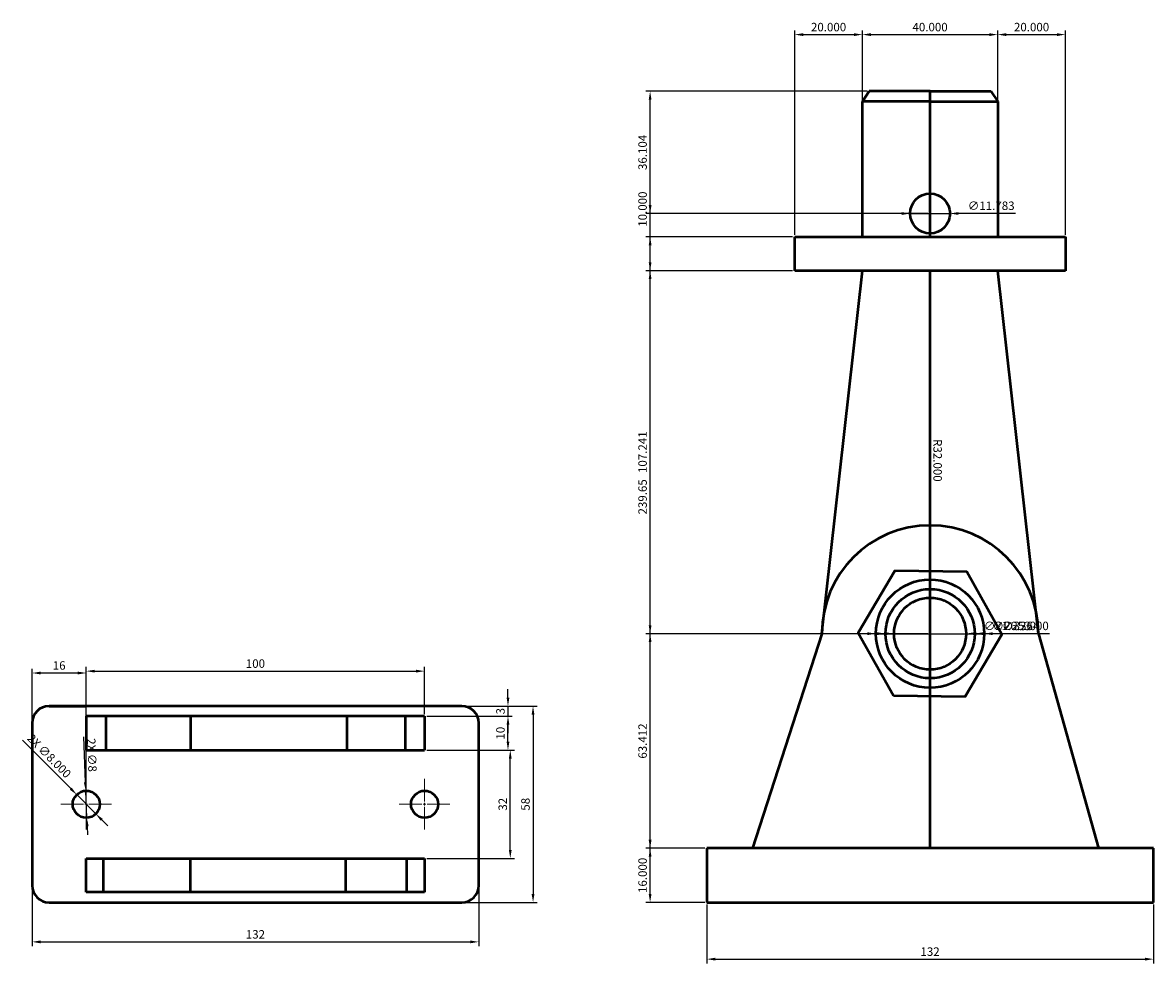
# Model space of a CAD drawing. Units: millimetres. Extents: x 1132 to 1696, y 1793 to 2376.
# Tile 3 of 4: x 1150 to 1484, y 2098 to 2376. Entities that reach past the tile are written whole.
import ezdxf

# ---------------------------------------------------------------- set-up
doc = ezdxf.new("R2010")
doc.units = ezdxf.units.MM
doc.linetypes.add('CENTER2', pattern=[28.575, 19.05, -3.175, 3.175, -3.175])
for name, color, linetype, lineweight in [('M-CNTR', 1, 'CENTER2', 18), ('M-DIMS', 2, 'Continuous', 25), ('M-OUTL', 7, 'Continuous', 50)]:
    doc.layers.add(name, color=color, linetype=linetype, lineweight=lineweight)
doc.styles.get("Standard").update_dxf_attribs({"font": 'arial.ttf'})
doc.dimstyles.new('ISO-25', dxfattribs={"dimtxt": 2.5, "dimasz": 2.5, "dimexe": 1.25, "dimexo": 0.625, "dimtad": 1, "dimtxsty": 'Standard', "dimcen": 2.5, "dimadec": 0, "dimazin": 0, "dimtfac": 1, "dimtmove": 0, "dimatfit": 3, "dimfxl": 1, "dimarcsym": 0})

# ---------------------------------------------------------------- blocks, each defined once
blk = doc.blocks.new('*D1')
at = {"layer": 'Defpoints', "color": 0, "transparency": 16777216}
for p in [(1152.81, 2120.87), (1284.81, 2120.87), (1284.81, 2104.21)]:
    blk.add_point(p, dxfattribs=at)
at = {"layer": 'M-DIMS', "color": 0, "lineweight": -2, "transparency": 16777216}
for p, q in [((1152.81, 2120.25), (1152.81, 2102.96)), ((1284.81, 2120.25), (1284.81, 2102.96)), ((1155.31, 2104.21), (1282.31, 2104.21))]:
    blk.add_line(p, q, dxfattribs=at)
at = {"layer": 'M-DIMS', "color": 0, "transparency": 16777216}
for points in [[(1155.31, 2104.63), (1155.31, 2103.79), (1152.81, 2104.21)], [(1282.31, 2104.63), (1282.31, 2103.79), (1284.81, 2104.21)]]:
    blk.add_solid(points, dxfattribs=at)
at = {"layer": 'M-DIMS', "color": 0, "transparency": 16777216, "insert": (1218.81, 2106.11), "char_height": 2.5, "attachment_point": 5}
blk.add_mtext('132', dxfattribs=at)
blk = doc.blocks.new('*D2')
at = {"layer": 'Defpoints', "color": 0, "transparency": 16777216}
for p in [(1279.81, 2173.87), (1279.81, 2115.87), (1300.87, 2115.87)]:
    blk.add_point(p, dxfattribs=at)
at = {"layer": 'M-DIMS', "color": 0, "lineweight": -2, "transparency": 16777216}
for p, q in [((1280.43, 2173.87), (1302.12, 2173.87)), ((1300.87, 2171.37), (1300.87, 2118.37)), ((1280.43, 2115.87), (1302.12, 2115.87))]:
    blk.add_line(p, q, dxfattribs=at)
at = {"layer": 'M-DIMS', "color": 0, "transparency": 16777216}
for points in [[(1300.45, 2171.37), (1301.28, 2171.37), (1300.87, 2173.87)], [(1300.45, 2118.37), (1301.28, 2118.37), (1300.87, 2115.87)]]:
    blk.add_solid(points, dxfattribs=at)
at = {"layer": 'M-DIMS', "color": 0, "transparency": 16777216, "insert": (1298.96, 2144.87), "char_height": 2.5, "attachment_point": 5, "rotation": 90}
blk.add_mtext('58', dxfattribs=at)
blk = doc.blocks.new('*D3')
at = {"layer": 'Defpoints', "color": 0, "transparency": 16777216}
for p in [(1268.81, 2160.87), (1294.14, 2160.87), (1268.81, 2128.87)]:
    blk.add_point(p, dxfattribs=at)
at = {"layer": 'M-DIMS', "color": 0, "lineweight": -2, "transparency": 16777216}
for p, q in [((1269.43, 2160.87), (1295.39, 2160.87)), ((1294.14, 2131.37), (1294.14, 2158.37)), ((1269.43, 2128.87), (1295.39, 2128.87))]:
    blk.add_line(p, q, dxfattribs=at)
at = {"layer": 'M-DIMS', "color": 0, "transparency": 16777216}
for points in [[(1293.72, 2158.37), (1294.55, 2158.37), (1294.14, 2160.87)], [(1293.72, 2131.37), (1294.55, 2131.37), (1294.14, 2128.87)]]:
    blk.add_solid(points, dxfattribs=at)
at = {"layer": 'M-DIMS', "color": 0, "transparency": 16777216, "insert": (1292.24, 2144.87), "char_height": 2.5, "attachment_point": 5, "rotation": 90}
blk.add_mtext('32', dxfattribs=at)
blk = doc.blocks.new('*D4')
at = {"layer": 'Defpoints', "color": 0, "transparency": 16777216}
for p in [(1268.81, 2170.87), (1293.46, 2170.87), (1268.81, 2160.87)]:
    blk.add_point(p, dxfattribs=at)
at = {"layer": 'M-DIMS', "color": 0, "lineweight": -2, "transparency": 16777216}
for p, q in [((1269.43, 2170.87), (1294.71, 2170.87)), ((1293.46, 2163.37), (1293.46, 2168.37)), ((1269.43, 2160.87), (1294.71, 2160.87))]:
    blk.add_line(p, q, dxfattribs=at)
at = {"layer": 'M-DIMS', "color": 0, "transparency": 16777216}
for points in [[(1293.05, 2168.37), (1293.88, 2168.37), (1293.46, 2170.87)], [(1293.05, 2163.37), (1293.88, 2163.37), (1293.46, 2160.87)]]:
    blk.add_solid(points, dxfattribs=at)
at = {"layer": 'M-DIMS', "color": 0, "transparency": 16777216, "insert": (1291.56, 2165.87), "char_height": 2.5, "attachment_point": 5, "rotation": 90}
blk.add_mtext('10', dxfattribs=at)
blk = doc.blocks.new('*D5')
at = {"layer": 'Defpoints', "color": 0, "transparency": 16777216}
for p in [(1279.81, 2173.87), (1282.07, 2170.87), (1293.46, 2170.87)]:
    blk.add_point(p, dxfattribs=at)
at = {"layer": 'M-DIMS', "color": 0, "lineweight": -2, "transparency": 16777216}
for p, q in [((1293.46, 2176.37), (1293.46, 2178.87)), ((1280.43, 2173.87), (1294.71, 2173.87)), ((1293.46, 2173.87), (1293.46, 2170.87)), ((1282.7, 2170.87), (1294.71, 2170.87)), ((1293.46, 2168.37), (1293.46, 2165.87))]:
    blk.add_line(p, q, dxfattribs=at)
at = {"layer": 'M-DIMS', "color": 0, "transparency": 16777216}
for points in [[(1293.05, 2176.37), (1293.88, 2176.37), (1293.46, 2173.87)], [(1293.05, 2168.37), (1293.88, 2168.37), (1293.46, 2170.87)]]:
    blk.add_solid(points, dxfattribs=at)
at = {"layer": 'M-DIMS', "color": 0, "transparency": 16777216, "insert": (1291.56, 2172.37), "char_height": 2.5, "attachment_point": 5, "rotation": 90}
blk.add_mtext('3', dxfattribs=at)
blk = doc.blocks.new('*D6')
at = {"layer": 'Defpoints', "color": 0, "transparency": 16777216}
for p in [(1268.81, 2184.2), (1168.81, 2170.87), (1268.81, 2170.87)]:
    blk.add_point(p, dxfattribs=at)
at = {"layer": 'M-DIMS', "color": 0, "lineweight": -2, "transparency": 16777216}
for p, q in [((1168.81, 2171.5), (1168.81, 2185.45)), ((1171.31, 2184.2), (1266.31, 2184.2)), ((1268.81, 2171.5), (1268.81, 2185.45))]:
    blk.add_line(p, q, dxfattribs=at)
at = {"layer": 'M-DIMS', "color": 0, "transparency": 16777216}
for points in [[(1171.31, 2184.61), (1171.31, 2183.78), (1168.81, 2184.2)], [(1266.31, 2184.61), (1266.31, 2183.78), (1268.81, 2184.2)]]:
    blk.add_solid(points, dxfattribs=at)
at = {"layer": 'M-DIMS', "color": 0, "transparency": 16777216, "insert": (1218.81, 2186.1), "char_height": 2.5, "attachment_point": 5}
blk.add_mtext('100', dxfattribs=at)
blk = doc.blocks.new('*D7')
at = {"layer": 'Defpoints', "color": 0, "transparency": 16777216}
for p in [(1152.81, 2183.65), (1152.81, 2144.87), (1168.81, 2144.87)]:
    blk.add_point(p, dxfattribs=at)
at = {"layer": 'M-DIMS', "color": 0, "lineweight": -2, "transparency": 16777216}
for p, q in [((1152.81, 2145.5), (1152.81, 2184.9)), ((1166.31, 2183.65), (1155.31, 2183.65)), ((1168.81, 2145.5), (1168.81, 2184.9))]:
    blk.add_line(p, q, dxfattribs=at)
at = {"layer": 'M-DIMS', "color": 0, "transparency": 16777216}
for points in [[(1155.31, 2184.06), (1155.31, 2183.23), (1152.81, 2183.65)], [(1166.31, 2184.06), (1166.31, 2183.23), (1168.81, 2183.65)]]:
    blk.add_solid(points, dxfattribs=at)
at = {"layer": 'M-DIMS', "color": 0, "transparency": 16777216, "insert": (1160.81, 2185.55), "char_height": 2.5, "attachment_point": 5}
blk.add_mtext('16', dxfattribs=at)
blk = doc.blocks.new('*U8')
at = {"layer": 'M-CNTR', "color": 0, "transparency": 16777216}
for p, q in [((0, 0.8), (0, 7.5)), ((-7.5, 0), (-0.8, 0)), ((0.8, 0), (7.5, 0)), ((0, -7.5), (0, -0.8))]:
    blk.add_line(p, q, dxfattribs=at)
at = {"layer": 'M-CNTR', "color": 0, "linetype": 'Continuous', "transparency": 16777216}
for p, q in [((-0.4, 0), (0.4, 0)), ((0, -0.4), (0, 0.4))]:
    blk.add_line(p, q, dxfattribs=at)
blk = doc.blocks.new('*U9')
at = {"layer": 'M-CNTR', "color": 0, "transparency": 16777216}
for p, q in [((0, 0.8), (0, 7.5)), ((-7.5, 0), (-0.8, 0)), ((0.8, 0), (7.5, 0)), ((0, -7.5), (0, -0.8))]:
    blk.add_line(p, q, dxfattribs=at)
at = {"layer": 'M-CNTR', "color": 0, "linetype": 'Continuous', "transparency": 16777216}
for p, q in [((-0.4, 0), (0.4, 0)), ((0, -0.4), (0, 0.4))]:
    blk.add_line(p, q, dxfattribs=at)
blk = doc.blocks.new('*D35')
at = {"layer": 'Defpoints', "color": 0, "transparency": 16777216}
for p in [(1352.22, 2115.86), (1484.22, 2115.86), (1484.22, 2099.11)]:
    blk.add_point(p, dxfattribs=at)
at = {"layer": 'M-DIMS', "color": 0, "lineweight": -2, "transparency": 16777216}
for p, q in [((1352.22, 2115.23), (1352.22, 2097.86)), ((1484.22, 2115.23), (1484.22, 2097.86)), ((1354.72, 2099.11), (1481.72, 2099.11))]:
    blk.add_line(p, q, dxfattribs=at)
at = {"layer": 'M-DIMS', "color": 0, "transparency": 16777216}
for points in [[(1354.72, 2099.53), (1354.72, 2098.69), (1352.22, 2099.11)], [(1481.72, 2099.53), (1481.72, 2098.69), (1484.22, 2099.11)]]:
    blk.add_solid(points, dxfattribs=at)
at = {"layer": 'M-DIMS', "color": 0, "transparency": 16777216, "insert": (1418.22, 2101.01), "char_height": 2.5, "attachment_point": 5}
blk.add_mtext('132', dxfattribs=at)
blk = doc.blocks.new('*D36')
at = {"layer": 'Defpoints', "color": 0, "transparency": 16777216}
for p in [(1335.47, 2355.51), (1400.22, 2355.51), (1352.22, 2115.86)]:
    blk.add_point(p, dxfattribs=at)
at = {"layer": 'M-DIMS', "color": 0, "lineweight": -2, "transparency": 16777216}
for p, q in [((1399.6, 2355.51), (1334.22, 2355.51)), ((1335.47, 2118.36), (1335.47, 2353.01)), ((1351.6, 2115.86), (1334.22, 2115.86))]:
    blk.add_line(p, q, dxfattribs=at)
at = {"layer": 'M-DIMS', "color": 0, "transparency": 16777216}
for points in [[(1335.06, 2353.01), (1335.89, 2353.01), (1335.47, 2355.51)], [(1335.06, 2118.36), (1335.89, 2118.36), (1335.47, 2115.86)]]:
    blk.add_solid(points, dxfattribs=at)
at = {"layer": 'M-DIMS', "color": 0, "transparency": 16777216, "insert": (1333.57, 2235.69), "char_height": 2.5, "attachment_point": 5, "rotation": 90}
blk.add_mtext('239.65', dxfattribs=at)
blk = doc.blocks.new('*D49')
at = {"layer": 'Defpoints', "color": 0, "transparency": 16777216}
for p in [(1168.64, 2148.87), (1168.98, 2140.88)]:
    blk.add_point(p, dxfattribs=at)
at = {"layer": 'M-DIMS', "color": 0, "lineweight": -2, "transparency": 16777216}
for p, q in [((1167.95, 2164.75), (1168.53, 2151.37)), ((1168.98, 2140.88), (1168.64, 2148.87)), ((1169.09, 2138.38), (1169.2, 2135.88))]:
    blk.add_line(p, q, dxfattribs=at)
at = {"layer": 'M-DIMS', "color": 0, "transparency": 16777216}
for points in [[(1168.94, 2151.39), (1168.11, 2151.35), (1168.64, 2148.87)], [(1169.51, 2138.4), (1168.68, 2138.36), (1168.98, 2140.88)]]:
    blk.add_solid(points, dxfattribs=at)
at = {"layer": 'M-DIMS', "color": 0, "transparency": 16777216, "insert": (1170.15, 2159.39), "char_height": 2.5, "attachment_point": 5, "rotation": 272.4898}
blk.add_mtext('2X ∅8', dxfattribs=at)
blk = doc.blocks.new('*D60')
at = {"layer": 'Defpoints', "color": 0, "transparency": 16777216}
for p in [(1335.47, 2131.86), (1352.22, 2131.86), (1352.22, 2115.86)]:
    blk.add_point(p, dxfattribs=at)
at = {"layer": 'M-DIMS', "color": 0, "lineweight": -2, "transparency": 16777216}
for p, q in [((1351.6, 2131.86), (1334.22, 2131.86)), ((1335.47, 2118.36), (1335.47, 2129.36)), ((1351.6, 2115.86), (1334.22, 2115.86))]:
    blk.add_line(p, q, dxfattribs=at)
at = {"layer": 'M-DIMS', "color": 0, "transparency": 16777216}
for points in [[(1335.06, 2129.36), (1335.89, 2129.36), (1335.47, 2131.86)], [(1335.06, 2118.36), (1335.89, 2118.36), (1335.47, 2115.86)]]:
    blk.add_solid(points, dxfattribs=at)
at = {"layer": 'M-DIMS', "color": 0, "transparency": 16777216, "insert": (1333.57, 2123.86), "char_height": 2.5, "attachment_point": 5, "rotation": 90}
blk.add_mtext('16.000', dxfattribs=at)
blk = doc.blocks.new('*D61')
at = {"layer": 'Defpoints', "color": 0, "transparency": 16777216}
for p in [(1335.47, 2195.27), (1418.22, 2195.27), (1352.22, 2131.86)]:
    blk.add_point(p, dxfattribs=at)
at = {"layer": 'M-DIMS', "color": 0, "lineweight": -2, "transparency": 16777216}
for p, q in [((1417.6, 2195.27), (1334.22, 2195.27)), ((1335.47, 2134.36), (1335.47, 2192.77)), ((1351.6, 2131.86), (1334.22, 2131.86))]:
    blk.add_line(p, q, dxfattribs=at)
at = {"layer": 'M-DIMS', "color": 0, "transparency": 16777216}
for points in [[(1335.06, 2192.77), (1335.89, 2192.77), (1335.47, 2195.27)], [(1335.06, 2134.36), (1335.89, 2134.36), (1335.47, 2131.86)]]:
    blk.add_solid(points, dxfattribs=at)
at = {"layer": 'M-DIMS', "color": 0, "transparency": 16777216, "insert": (1333.57, 2163.56), "char_height": 2.5, "attachment_point": 5, "rotation": 90}
blk.add_mtext('63.412', dxfattribs=at)
blk = doc.blocks.new('*D62')
at = {"layer": 'Defpoints', "color": 0, "transparency": 16777216}
for p in [(1335.47, 2302.51), (1378.22, 2302.51), (1418.22, 2195.27)]:
    blk.add_point(p, dxfattribs=at)
at = {"layer": 'M-DIMS', "color": 0, "lineweight": -2, "transparency": 16777216}
for p, q in [((1377.6, 2302.51), (1334.22, 2302.51)), ((1335.47, 2197.77), (1335.47, 2300.01)), ((1417.6, 2195.27), (1334.22, 2195.27))]:
    blk.add_line(p, q, dxfattribs=at)
at = {"layer": 'M-DIMS', "color": 0, "transparency": 16777216}
for points in [[(1335.06, 2300.01), (1335.89, 2300.01), (1335.47, 2302.51)], [(1335.06, 2197.77), (1335.89, 2197.77), (1335.47, 2195.27)]]:
    blk.add_solid(points, dxfattribs=at)
at = {"layer": 'M-DIMS', "color": 0, "transparency": 16777216, "insert": (1333.57, 2248.89), "char_height": 2.5, "attachment_point": 5, "rotation": 90}
blk.add_mtext('107.241', dxfattribs=at)
blk = doc.blocks.new('*D63')
at = {"layer": 'Defpoints', "color": 0, "transparency": 16777216}
for p in [(1335.47, 2312.51), (1378.22, 2312.51), (1378.22, 2302.51)]:
    blk.add_point(p, dxfattribs=at)
at = {"layer": 'M-DIMS', "color": 0, "lineweight": -2, "transparency": 16777216}
for p, q in [((1335.47, 2312.51), (1335.47, 2326.4)), ((1377.6, 2312.51), (1334.22, 2312.51)), ((1335.47, 2305.01), (1335.47, 2310.01)), ((1377.6, 2302.51), (1334.22, 2302.51))]:
    blk.add_line(p, q, dxfattribs=at)
at = {"layer": 'M-DIMS', "color": 0, "transparency": 16777216}
for points in [[(1335.06, 2310.01), (1335.89, 2310.01), (1335.47, 2312.51)], [(1335.06, 2305.01), (1335.89, 2305.01), (1335.47, 2302.51)]]:
    blk.add_solid(points, dxfattribs=at)
at = {"layer": 'M-DIMS', "color": 0, "transparency": 16777216, "insert": (1333.57, 2320.7), "char_height": 2.5, "attachment_point": 5, "rotation": 90}
blk.add_mtext('10.000', dxfattribs=at)
blk = doc.blocks.new('*D64')
at = {"layer": 'Defpoints', "color": 0, "transparency": 16777216}
for p in [(1335.47, 2355.51), (1400.22, 2355.51), (1418.22, 2319.41)]:
    blk.add_point(p, dxfattribs=at)
at = {"layer": 'M-DIMS', "color": 0, "lineweight": -2, "transparency": 16777216}
for p, q in [((1399.6, 2355.51), (1334.22, 2355.51)), ((1335.47, 2321.91), (1335.47, 2353.01)), ((1417.6, 2319.41), (1334.22, 2319.41))]:
    blk.add_line(p, q, dxfattribs=at)
at = {"layer": 'M-DIMS', "color": 0, "transparency": 16777216}
for points in [[(1335.06, 2353.01), (1335.89, 2353.01), (1335.47, 2355.51)], [(1335.06, 2321.91), (1335.89, 2321.91), (1335.47, 2319.41)]]:
    blk.add_solid(points, dxfattribs=at)
at = {"layer": 'M-DIMS', "color": 0, "transparency": 16777216, "insert": (1333.57, 2337.46), "char_height": 2.5, "attachment_point": 5, "rotation": 90}
blk.add_mtext('36.104', dxfattribs=at)
blk = doc.blocks.new('*D65')
at = {"layer": 'Defpoints', "color": 0, "transparency": 16777216}
for p in [(1398.22, 2372.26), (1378.22, 2312.51), (1398.22, 2312.51)]:
    blk.add_point(p, dxfattribs=at)
at = {"layer": 'M-DIMS', "color": 0, "lineweight": -2, "transparency": 16777216}
for p, q in [((1378.22, 2313.14), (1378.22, 2373.51)), ((1398.22, 2313.14), (1398.22, 2373.51)), ((1380.72, 2372.26), (1395.72, 2372.26))]:
    blk.add_line(p, q, dxfattribs=at)
at = {"layer": 'M-DIMS', "color": 0, "transparency": 16777216}
for points in [[(1380.72, 2372.68), (1380.72, 2371.84), (1378.22, 2372.26)], [(1395.72, 2372.68), (1395.72, 2371.84), (1398.22, 2372.26)]]:
    blk.add_solid(points, dxfattribs=at)
at = {"layer": 'M-DIMS', "color": 0, "transparency": 16777216, "insert": (1388.22, 2374.16), "char_height": 2.5, "attachment_point": 5}
blk.add_mtext('20.000', dxfattribs=at)
blk = doc.blocks.new('*D66')
at = {"layer": 'Defpoints', "color": 0, "transparency": 16777216}
for p in [(1438.22, 2372.26), (1398.22, 2312.51), (1438.22, 2312.51)]:
    blk.add_point(p, dxfattribs=at)
at = {"layer": 'M-DIMS', "color": 0, "lineweight": -2, "transparency": 16777216}
for p, q in [((1398.22, 2313.14), (1398.22, 2373.51)), ((1438.22, 2313.14), (1438.22, 2373.51)), ((1400.72, 2372.26), (1435.72, 2372.26))]:
    blk.add_line(p, q, dxfattribs=at)
at = {"layer": 'M-DIMS', "color": 0, "transparency": 16777216}
for points in [[(1400.72, 2372.68), (1400.72, 2371.84), (1398.22, 2372.26)], [(1435.72, 2372.68), (1435.72, 2371.84), (1438.22, 2372.26)]]:
    blk.add_solid(points, dxfattribs=at)
at = {"layer": 'M-DIMS', "color": 0, "transparency": 16777216, "insert": (1418.22, 2374.16), "char_height": 2.5, "attachment_point": 5}
blk.add_mtext('40.000', dxfattribs=at)
blk = doc.blocks.new('*D67')
at = {"layer": 'Defpoints', "color": 0, "transparency": 16777216}
for p in [(1458.22, 2372.26), (1438.22, 2312.51), (1458.22, 2312.51)]:
    blk.add_point(p, dxfattribs=at)
at = {"layer": 'M-DIMS', "color": 0, "lineweight": -2, "transparency": 16777216}
for p, q in [((1438.22, 2313.14), (1438.22, 2373.51)), ((1458.22, 2313.14), (1458.22, 2373.51)), ((1440.72, 2372.26), (1455.72, 2372.26))]:
    blk.add_line(p, q, dxfattribs=at)
at = {"layer": 'M-DIMS', "color": 0, "transparency": 16777216}
for points in [[(1440.72, 2372.68), (1440.72, 2371.84), (1438.22, 2372.26)], [(1455.72, 2372.68), (1455.72, 2371.84), (1458.22, 2372.26)]]:
    blk.add_solid(points, dxfattribs=at)
at = {"layer": 'M-DIMS', "color": 0, "transparency": 16777216, "insert": (1448.22, 2374.16), "char_height": 2.5, "attachment_point": 5}
blk.add_mtext('20.000', dxfattribs=at)
blk = doc.blocks.new('*D78')
at = {"layer": 'Defpoints', "color": 0, "transparency": 16777216}
for p in [(1402.22, 2195.27), (1434.22, 2195.27)]:
    blk.add_point(p, dxfattribs=at)
at = {"layer": 'M-DIMS', "color": 0, "lineweight": -2, "transparency": 16777216}
for p, q in [((1399.72, 2195.27), (1397.22, 2195.27)), ((1402.22, 2195.27), (1434.22, 2195.27)), ((1453.56, 2195.27), (1436.72, 2195.27))]:
    blk.add_line(p, q, dxfattribs=at)
at = {"layer": 'M-DIMS', "color": 0, "transparency": 16777216}
for points in [[(1399.72, 2195.69), (1399.72, 2194.85), (1402.22, 2195.27)], [(1436.72, 2195.69), (1436.72, 2194.85), (1434.22, 2195.27)]]:
    blk.add_solid(points, dxfattribs=at)
at = {"layer": 'M-DIMS', "color": 0, "transparency": 16777216, "insert": (1446.39, 2197.24), "char_height": 2.5, "attachment_point": 5, "rotation": 0.0009}
blk.add_mtext('∅32.000', dxfattribs=at)
blk = doc.blocks.new('*D79')
at = {"layer": 'Defpoints', "color": 0, "transparency": 16777216}
for p in [(1405.04, 2195.27), (1431.41, 2195.27)]:
    blk.add_point(p, dxfattribs=at)
at = {"layer": 'M-DIMS', "color": 0, "lineweight": -2, "transparency": 16777216}
for p, q in [((1402.54, 2195.27), (1400.04, 2195.27)), ((1405.04, 2195.27), (1431.41, 2195.27)), ((1450.74, 2195.27), (1433.91, 2195.27))]:
    blk.add_line(p, q, dxfattribs=at)
at = {"layer": 'M-DIMS', "color": 0, "transparency": 16777216}
for points in [[(1402.54, 2195.69), (1402.54, 2194.85), (1405.04, 2195.27)], [(1433.91, 2195.69), (1433.91, 2194.85), (1431.41, 2195.27)]]:
    blk.add_solid(points, dxfattribs=at)
at = {"layer": 'M-DIMS', "color": 0, "transparency": 16777216, "insert": (1443.58, 2197.24), "char_height": 2.5, "attachment_point": 5, "rotation": 0.0011}
blk.add_mtext('∅26.364', dxfattribs=at)
blk = doc.blocks.new('*D80')
at = {"layer": 'Defpoints', "color": 0, "transparency": 16777216}
for p in [(1407.6, 2195.27), (1428.85, 2195.27)]:
    blk.add_point(p, dxfattribs=at)
at = {"layer": 'M-DIMS', "color": 0, "lineweight": -2, "transparency": 16777216}
for p, q in [((1405.1, 2195.27), (1402.6, 2195.27)), ((1407.6, 2195.27), (1428.85, 2195.27)), ((1448.2, 2195.27), (1431.35, 2195.27))]:
    blk.add_line(p, q, dxfattribs=at)
at = {"layer": 'M-DIMS', "color": 0, "transparency": 16777216}
for points in [[(1405.1, 2195.69), (1405.1, 2194.85), (1407.6, 2195.27)], [(1431.35, 2195.69), (1431.35, 2194.85), (1428.85, 2195.27)]]:
    blk.add_solid(points, dxfattribs=at)
at = {"layer": 'M-DIMS', "color": 0, "transparency": 16777216, "insert": (1441.03, 2197.24), "char_height": 2.5, "attachment_point": 5, "rotation": 0.0014}
blk.add_mtext('∅21.253', dxfattribs=at)
blk = doc.blocks.new('*D81')
at = {"layer": 'Defpoints', "color": 0, "transparency": 16777216}
for p in [(1418.22, 2227.27), (1418.22, 2195.27)]:
    blk.add_point(p, dxfattribs=at)
at = {"layer": 'M-DIMS', "color": 0, "lineweight": -2, "transparency": 16777216}
for p, q in [((1418.22, 2253.48), (1418.22, 2229.77)), ((1418.22, 2195.27), (1418.22, 2227.27))]:
    blk.add_line(p, q, dxfattribs=at)
at = {"layer": 'M-DIMS', "color": 0, "transparency": 16777216}
blk.add_solid([(1418.64, 2229.77), (1417.81, 2229.77), (1418.22, 2227.27)], dxfattribs=at)
at = {"layer": 'M-DIMS', "color": 0, "transparency": 16777216, "insert": (1420.13, 2246.47), "char_height": 2.5, "attachment_point": 5, "rotation": 270.0006}
blk.add_mtext('R32.000', dxfattribs=at)
blk = doc.blocks.new('*D82')
at = {"layer": 'Defpoints', "color": 0, "transparency": 16777216}
for p in [(1412.33, 2319.41), (1424.12, 2319.41)]:
    blk.add_point(p, dxfattribs=at)
at = {"layer": 'M-DIMS', "color": 0, "lineweight": -2, "transparency": 16777216}
for p, q in [((1409.83, 2319.41), (1407.33, 2319.41)), ((1412.33, 2319.41), (1424.12, 2319.41)), ((1443.46, 2319.41), (1426.62, 2319.41))]:
    blk.add_line(p, q, dxfattribs=at)
at = {"layer": 'M-DIMS', "color": 0, "transparency": 16777216}
for points in [[(1409.83, 2319.82), (1409.83, 2318.99), (1412.33, 2319.41)], [(1426.62, 2319.82), (1426.62, 2318.99), (1424.12, 2319.41)]]:
    blk.add_solid(points, dxfattribs=at)
at = {"layer": 'M-DIMS', "color": 0, "transparency": 16777216, "insert": (1436.29, 2321.38), "char_height": 2.5, "attachment_point": 5, "rotation": 359.9958}
blk.add_mtext('∅11.783', dxfattribs=at)
blk = doc.blocks.new('*D83')
at = {"layer": 'Defpoints', "color": 0, "transparency": 16777216}
for p in [(1165.99, 2147.71), (1171.63, 2142.04)]:
    blk.add_point(p, dxfattribs=at)
at = {"layer": 'M-DIMS', "color": 0, "lineweight": -2, "transparency": 16777216}
for p, q in [((1150, 2163.79), (1164.23, 2149.48)), ((1171.63, 2142.04), (1165.99, 2147.71)), ((1173.39, 2140.26), (1175.16, 2138.49))]:
    blk.add_line(p, q, dxfattribs=at)
at = {"layer": 'M-DIMS', "color": 0, "transparency": 16777216}
for points in [[(1164.52, 2149.78), (1163.93, 2149.19), (1165.99, 2147.71)], [(1173.69, 2140.56), (1173.1, 2139.97), (1171.63, 2142.04)]]:
    blk.add_solid(points, dxfattribs=at)
at = {"layer": 'M-DIMS', "color": 0, "transparency": 16777216, "insert": (1157.63, 2158.91), "char_height": 2.5, "attachment_point": 5, "rotation": 314.8321}
blk.add_mtext('2X ∅8.000', dxfattribs=at)

msp = doc.modelspace()

# ---------------------------------------------------------------- linework, layer by layer
at = {"layer": 'M-OUTL'}
for p, q in [((1398.2243, 2352.5114), (1400.2243, 2355.5114)), ((1418.2243, 2355.5114), (1400.2243, 2355.5114)), ((1418.2243, 2352.5114), (1418.2243, 2355.5114)), ((1418.2243, 2355.5114), (1436.2243, 2355.5114)), ((1436.2243, 2355.5114), (1438.2243, 2352.5114)), ((1398.2243, 2312.5114), (1398.2243, 2352.5114)), ((1418.2243, 2352.5114), (1398.2243, 2352.5114)), ((1418.2243, 2352.5114), (1438.2243, 2352.5114)), ((1418.2243, 2319.4074), (1418.2243, 2352.5114)), ((1438.2243, 2352.5114), (1438.2243, 2312.5114)), ((1418.2243, 2312.5114), (1418.2243, 2319.4074)), ((1378.2243, 2302.5114), (1378.2243, 2312.5114)), ((1378.2243, 2312.5114), (1458.2243, 2312.5114)), ((1458.2243, 2312.5114), (1458.2243, 2302.5114)), ((1418.2243, 2302.5114), (1378.2243, 2302.5114)), ((1386.2243, 2195.2707), (1398.2243, 2302.5114)), ((1418.2243, 2195.2707), (1418.2243, 2302.5114)), ((1458.2243, 2302.5114), (1418.2243, 2302.5114)), ((1450.2243, 2195.2707), (1438.2243, 2302.5114)), ((1386.2243, 2195.2707), (1365.6966, 2131.8589)), ((1418.2243, 2131.8589), (1418.2243, 2195.2707)), ((1450.2243, 2195.2707), (1467.9922, 2131.8589)), ((1279.8099, 2173.8736), (1157.8099, 2173.8736)), ((1157.8099, 2173.8736), (1168.8099, 2173.8736)), ((1279.8099, 2173.8736), (1268.8099, 2173.8736)), ((1268.8099, 2170.8736), (1168.8099, 2170.8736)), ((1168.8099, 2170.8736), (1168.8099, 2160.8736)), ((1174.5593, 2170.8736), (1174.5593, 2160.8736)), ((1199.626, 2170.8736), (1199.626, 2160.8736)), ((1245.8359, 2170.8736), (1245.8359, 2160.8736)), ((1263.0556, 2170.8736), (1263.0556, 2160.8736)), ((1268.8099, 2170.8736), (1268.8099, 2160.8736)), ((1152.8099, 2168.8736), (1152.8099, 2120.8736)), ((1284.8099, 2120.8736), (1284.8099, 2168.8736)), ((1168.8099, 2160.8736), (1268.8099, 2160.8736)), ((1484.2243, 2131.8589), (1352.2243, 2131.8589)), ((1352.2243, 2131.8589), (1352.2243, 2115.8589)), ((1484.2243, 2115.8589), (1484.2243, 2131.8589)), ((1168.8099, 2118.8736), (1168.8099, 2128.8736)), ((1168.8099, 2128.8736), (1268.8099, 2128.8736)), ((1173.9054, 2118.8736), (1173.9054, 2128.8736)), ((1199.626, 2118.8736), (1199.626, 2128.8736)), ((1245.4, 2128.8736), (1245.4, 2118.8736)), ((1263.4916, 2128.8736), (1263.4916, 2118.8736)), ((1268.8099, 2128.8736), (1268.8099, 2118.8736)), ((1157.8099, 2115.8736), (1279.8099, 2115.8736)), ((1268.8099, 2118.8736), (1168.8099, 2118.8736)), ((1352.2243, 2115.8589), (1484.2243, 2115.8589))]:
    msp.add_line(p, q, dxfattribs=at)
msp.add_lwpolyline([(1407.3769, 2176.9943), (1428.6285, 2176.7383), (1439.4759, 2195.0148), (1429.0718, 2213.5472), (1407.8202, 2213.8032), (1396.9727, 2195.5267)], close=True, dxfattribs=at)
for centre, radius in [((1418.2243, 2319.4074), 5.8916), ((1418.2243, 2195.2707), 16), ((1418.2243, 2195.2707), 13.1819), ((1418.2243, 2195.2707), 10.6266), ((1168.8099, 2144.8736), 4), ((1268.8099, 2144.8736), 4)]:
    msp.add_circle(centre, radius, dxfattribs=at)
for centre, radius, start, end in [((1418.2243, 2195.2707), 32, 0, 180), ((1157.8099, 2168.8736), 5, 90, 180), ((1279.8099, 2168.8736), 5, 0, 90), ((1157.8099, 2120.8736), 5, 180, 270), ((1279.8099, 2120.8736), 5, 270, 0)]:
    msp.add_arc(centre, radius, start, end, dxfattribs=at)

# ---------------------------------------------------------------- block references
at = {"layer": 'M-CNTR'}
for name, p in [('*U8', (1168.8099, 2144.8736)), ('*U9', (1268.8099, 2144.8736))]:
    msp.add_blockref(name, p, dxfattribs=at)

# ---------------------------------------------------------------- dimensions: what is measured, and where the dimension line sits
at = {"layer": 'M-DIMS'}
for base, p1, p2, override, picture, middle in [((1398.2243, 2372.2614), (1378.2243, 2312.5114), (1398.2243, 2312.5114), {"dimdec": 3, "dimlfac": 1, "dimrnd": 0, "dimzin": 0, "dimdsep": 46, "dimlunit": 2}, '*D65', (1388.2243, 2374.1629)), ((1438.2243, 2372.2614), (1398.2243, 2312.5114), (1438.2243, 2312.5114), {"dimdec": 3, "dimlfac": 1, "dimrnd": 0, "dimzin": 0, "dimdsep": 46, "dimlunit": 2}, '*D66', (1418.2243, 2374.1629)), ((1458.2243, 2372.2614), (1438.2243, 2312.5114), (1458.2243, 2312.5114), {"dimdec": 3, "dimlfac": 1, "dimrnd": 0, "dimzin": 0, "dimdsep": 46, "dimlunit": 2}, '*D67', (1448.2243, 2374.1629)), ((1152.8099, 2183.6456), (1168.8099, 2144.8736), (1152.8099, 2144.8736), {"dimclrd": 0, "dimclre": 0, "dimclrt": 0}, '*D7', (1160.8099, 2185.547)), ((1268.8099, 2184.1953), (1168.8099, 2170.8736), (1268.8099, 2170.8736), {"dimclrd": 0, "dimclre": 0, "dimclrt": 0}, '*D6', (1218.8099, 2186.0967)), ((1284.8099, 2104.2101), (1152.8099, 2120.8736), (1284.8099, 2120.8736), {"dimclrd": 0, "dimclre": 0, "dimclrt": 0}, '*D1', (1218.8099, 2106.1123)), ((1484.2243, 2099.1089), (1352.2243, 2115.8589), (1484.2243, 2115.8589), {"dimdec": 0, "dimlfac": 1, "dimrnd": 0, "dimzin": 0, "dimdsep": 46, "dimlunit": 2}, '*D35', (1418.2243, 2101.0112))]:
    dim = msp.add_linear_dim(base=base, p1=p1, p2=p2, dimstyle='ISO-25', override=override, dxfattribs=at)
    dim.commit()
    dim.dimension.update_dxf_attribs({"geometry": picture, "text_midpoint": middle})
for base, p1, p2, override, picture, middle in [((1335.4743, 2355.5114), (1352.2243, 2115.8589), (1400.2243, 2355.5114), {"dimdec": 2, "dimlfac": 1, "dimrnd": 0, "dimzin": 0, "dimdsep": 46, "dimlunit": 2}, '*D36', (1333.572, 2235.6852)), ((1335.4743, 2355.5114), (1418.2243, 2319.4074), (1400.2243, 2355.5114), {"dimdec": 3, "dimlfac": 1, "dimrnd": 0, "dimzin": 0, "dimdsep": 46, "dimlunit": 2}, '*D64', (1333.572, 2337.4594)), ((1335.4743, 2312.5114), (1378.2243, 2302.5114), (1378.2243, 2312.5114), {"dimdec": 3, "dimlfac": 1, "dimrnd": 0, "dimzin": 0, "dimdsep": 46, "dimlunit": 2}, '*D63', (1333.5729, 2320.7038)), ((1335.4743, 2302.5114), (1418.2243, 2195.2707), (1378.2243, 2302.5114), {"dimdec": 3, "dimlfac": 1, "dimrnd": 0, "dimzin": 0, "dimdsep": 46, "dimlunit": 2}, '*D62', (1333.5729, 2248.8911)), ((1335.4743, 2195.2707), (1352.2243, 2131.8589), (1418.2243, 2195.2707), {"dimdec": 3, "dimlfac": 1, "dimrnd": 0, "dimzin": 0, "dimdsep": 46, "dimlunit": 2}, '*D61', (1333.572, 2163.5648)), ((1293.4645, 2170.8736), (1279.8099, 2173.8736), (1282.0747, 2170.8736), {"dimclrd": 0, "dimclre": 0, "dimclrt": 0}, '*D5', (1291.5622, 2172.3736)), ((1300.866, 2115.8736), (1279.8099, 2173.8736), (1279.8099, 2115.8736), {"dimclrd": 0, "dimclre": 0, "dimclrt": 0}, '*D2', (1298.9646, 2144.8736)), ((1293.4645, 2170.8736), (1268.8099, 2160.8736), (1268.8099, 2170.8736), {"dimclrd": 0, "dimclre": 0, "dimclrt": 0}, '*D4', (1291.563, 2165.8736)), ((1294.1373, 2160.8736), (1268.8099, 2128.8736), (1268.8099, 2160.8736), {"dimclrd": 0, "dimclre": 0, "dimclrt": 0}, '*D3', (1292.235, 2144.8736)), ((1335.4743, 2131.8589), (1352.2243, 2115.8589), (1352.2243, 2131.8589), {"dimdec": 3, "dimlfac": 1, "dimrnd": 0, "dimzin": 0, "dimdsep": 46, "dimlunit": 2}, '*D60', (1333.5729, 2123.8589))]:
    dim = msp.add_linear_dim(base=base, p1=p1, p2=p2, angle=90, dimstyle='ISO-25', override=override, dxfattribs=at)
    dim.commit()
    dim.dimension.update_dxf_attribs({"geometry": picture, "text_midpoint": middle})
for p1, p2, picture, middle in [((1412.3327, 2319.4079), (1424.1159, 2319.407), '*D82', (1436.2902, 2319.4061)), ((1402.2243, 2195.2705), (1434.2243, 2195.271), '*D78', (1446.3943, 2195.2712)), ((1405.0424, 2195.2705), (1431.4062, 2195.271), '*D79', (1443.5754, 2195.2712)), ((1407.5977, 2195.2705), (1428.8509, 2195.271), '*D80', (1441.0252, 2195.2713))]:
    dim = msp.add_diameter_dim_2p(p1=p1, p2=p2, dimstyle='ISO-25', override={"dimdec": 3, "dimlfac": 1, "dimrnd": 0, "dimzin": 0, "dimdsep": 46, "dimlunit": 2}, dxfattribs=at)
    dim.commit()
    dim.dimension.update_dxf_attribs({"geometry": picture, "text_midpoint": middle})
dim = msp.add_radius_dim(center=(1418.2243, 2195.2707), mpoint=(1418.224, 2227.2707), dimstyle='ISO-25', override={"dimdec": 3, "dimlfac": 1, "dimrnd": 0, "dimzin": 0, "dimdsep": 46, "dimlunit": 2}, dxfattribs=at)
dim.commit()
dim.dimension.update_dxf_attribs({"geometry": '*D81', "text_midpoint": (1418.2238, 2246.4707), "dimtype": 164})
for p1, p2, override, picture, middle in [((1171.63, 2142.0369), (1165.9897, 2147.7103), {"dimdec": 3, "dimlfac": 1, "dimrnd": 0, "dimzin": 0, "dimdsep": 46, "dimlunit": 2}, '*D83', (1156.2324, 2157.525)), ((1168.9836, 2140.8774), (1168.6361, 2148.8698), {"dimdec": 0, "dimlfac": 1, "dimrnd": 0, "dimzin": 0, "dimdsep": 46, "dimlunit": 2}, '*D49', (1168.1822, 2159.3076))]:
    dim = msp.add_diameter_dim_2p(p1=p1, p2=p2, text='2X <>', dimstyle='ISO-25', override=override, dxfattribs=at)
    dim.commit()
    dim.dimension.update_dxf_attribs({"geometry": picture, "text_midpoint": middle})

doc.saveas('drawing.dxf')
